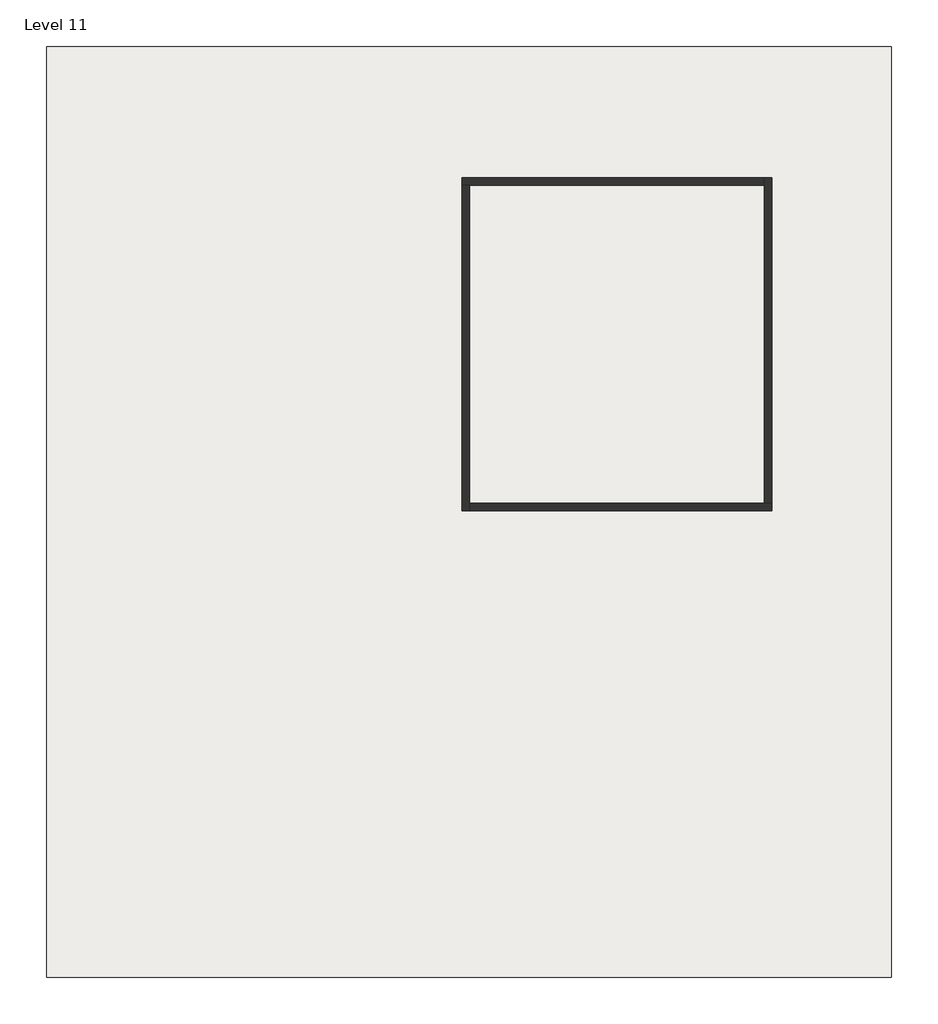
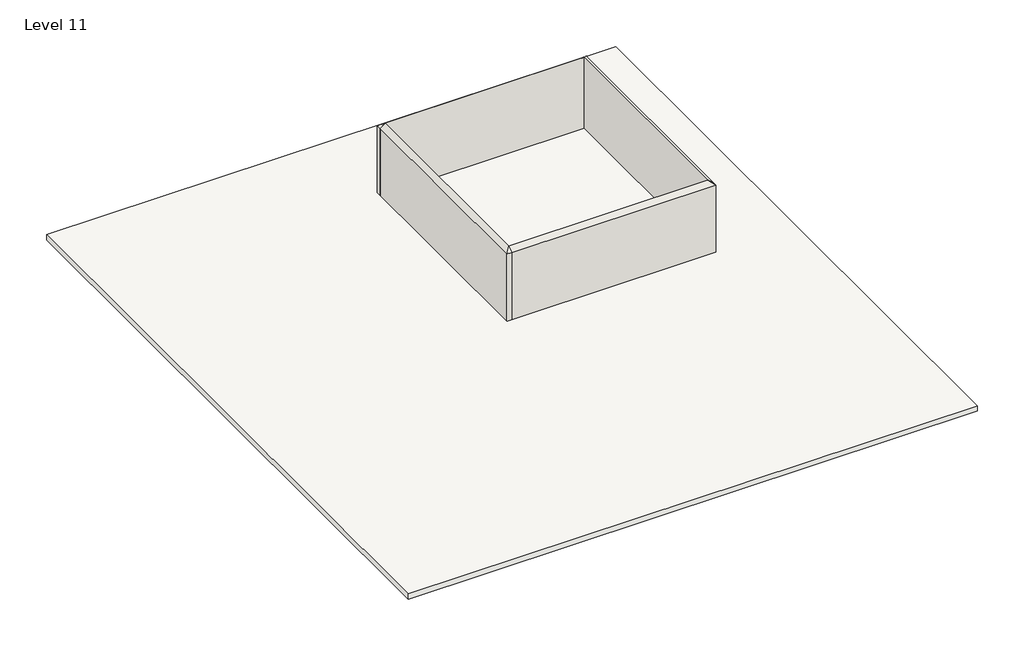
# One storey, incomplete: 4 walls, 1 roof.
"""IFC4 building model written with IfcOpenShell, lengths in millimetres."""

from ifc_helpers import new_model, si_unit, frame, origin, place, context, project, spatial, polyline, outline, extrude, faceted_brep, element, save

model = new_model("IFC4")

# Units and contexts
model_context = context("Model", 3, world=origin())
ifc_project = project(units=[si_unit("LENGTHUNIT", "METRE", prefix="MILLI")], contexts=[model_context])

# Site, building, storey
site = spatial("IfcSite", under=ifc_project)
building = spatial("IfcBuilding", under=site)
storey = spatial("IfcBuildingStorey", under=building, Name="Level 11", Elevation=12877.8)

# Roof
placement = place(None, origin())
element("IfcRoof", 1, ObjectType="Generic - 9\"", at=placement, inside=storey, context=model_context, shape_type="SweptSolid", body=[
    extrude(outline(polyline([(-11268.6561094, 14639.671536), (11286.5438906, 14639.671536), (11286.5438906, -10201.528464), (-11268.6561094, -10201.528464), (-11268.6561094, 14639.671536)])), frame((0.0, 0.0, 12877.8), z_axis=(0.0, 0.0, 1.0), x_axis=(1.0, 0.0, 0.0)), (0.0, 0.0, 1.0), 228.6),
])

# Walls
element("IfcWall", 2, ObjectType="Generic - 8\"", at=placement, inside=storey, context=model_context, shape_type="Brep", body=[
    faceted_brep([(-177.9928125, 10938.7037429, 12877.8), (25.2071875, 10938.7037429, 12877.8), (7899.2071875, 10938.7037429, 12877.8), (7899.2071875, 10938.7037429, 16078.2), (25.2071875, 10938.7037429, 16078.2), (-177.9928125, 10938.7037429, 15925.8), (-177.9928125, 11141.9037429, 12877.8), (-177.9928125, 11141.9037429, 15925.8), (7899.2071875, 11141.9037429, 15925.8), (7899.2071875, 11141.9037429, 12877.8)], [[[0, 1, 2, 3, 4, 5]], [[6, 7, 8, 9]], [[2, 1, 0, 6, 9]], [[0, 5, 7, 6]], [[3, 2, 9, 8]], [[5, 4, 7]], [[4, 3, 8, 7]]]),
])
element("IfcWall", 3, ObjectType="Generic - 8\"", at=placement, inside=storey, context=model_context, shape_type="Brep", body=[
    faceted_brep([(25.2071875, 2251.9037429, 12877.8), (25.2071875, 2455.1037429, 12877.8), (25.2071875, 10938.7037429, 12877.8), (25.2071875, 10938.7037429, 16078.2), (25.2071875, 2455.1037429, 16078.2), (25.2071875, 2251.9037429, 15925.8), (-177.9928125, 2251.9037429, 12877.8), (-177.9928125, 2251.9037429, 15925.8), (-177.9928125, 10938.7037429, 15925.8), (-177.9928125, 10938.7037429, 12877.8)], [[[0, 1, 2, 3, 4, 5]], [[6, 7, 8, 9]], [[2, 1, 0, 6, 9]], [[0, 5, 7, 6]], [[3, 2, 9, 8]], [[5, 4, 7]], [[4, 3, 8, 7]]]),
])
element("IfcWall", 4, ObjectType="Generic - 8\"", at=placement, inside=storey, context=model_context, shape_type="Brep", body=[
    faceted_brep([(8102.4071875, 2455.1037429, 12877.8), (7899.2071875, 2455.1037429, 12877.8), (25.2071875, 2455.1037429, 12877.8), (25.2071875, 2455.1037429, 16078.2), (7899.2071875, 2455.1037429, 16078.2), (8102.4071875, 2455.1037429, 15925.8), (8102.4071875, 2251.9037429, 12877.8), (8102.4071875, 2251.9037429, 15925.8), (25.2071875, 2251.9037429, 15925.8), (25.2071875, 2251.9037429, 12877.8)], [[[0, 1, 2, 3, 4, 5]], [[6, 7, 8, 9]], [[2, 1, 0, 6, 9]], [[0, 5, 7, 6]], [[3, 2, 9, 8]], [[5, 4, 7]], [[4, 3, 8, 7]]]),
])
element("IfcWall", 5, ObjectType="Generic - 8\"", at=placement, inside=storey, context=model_context, shape_type="Brep", body=[
    faceted_brep([(7899.2071875, 11141.9037429, 12877.8), (7899.2071875, 10938.7037429, 12877.8), (7899.2071875, 2455.1037429, 12877.8), (7899.2071875, 2455.1037429, 16078.2), (7899.2071875, 10938.7037429, 16078.2), (7899.2071875, 11141.9037429, 15925.8), (8102.4071875, 11141.9037429, 12877.8), (8102.4071875, 11141.9037429, 15925.8), (8102.4071875, 2455.1037429, 15925.8), (8102.4071875, 2455.1037429, 12877.8)], [[[0, 1, 2, 3, 4, 5]], [[6, 7, 8, 9]], [[2, 1, 0, 6, 9]], [[0, 5, 7, 6]], [[3, 2, 9, 8]], [[5, 4, 7]], [[4, 3, 8, 7]]]),
])

save(model, "model.ifc")

# Revit data of these elements
# Type "Generic - 9\""
#   Assembly Code = "B1020"
#   Layers, outside or top first: 0' - 9" no material (function 1)
# Type "Generic - 8\""
#   Assembly Code = "B2010"
#   Layers, outside or top first: 0' - 8" no material (function 1)
# Element 1 (IfcRoof, "Generic - 9\"")
#   built-in parameter 1001705 = 43 (stored number, unit not read)
#   built-in parameter 1001710 = 33615
#   Phase Created = New Construction
#   Materials on its faces: "Default Roof"
# Elements 2, 3, 4, 5 (IfcWall, "Generic - 8\"")
#   Top Offset = 0' - 0"
#   Base Offset = 0' - 0"
#   Unconnected Height = 10' - 0"
#   wall height = 10' - 0"
#   Phase Created = New Construction
#   Base Constraint = Level 11
#   Materials on its faces: "Default Wall"
# Materials
#   "Default Roof": colour RGB 88 101 114, transparency 0
#   "Default Wall": colour RGB 128 128 128, transparency 0
